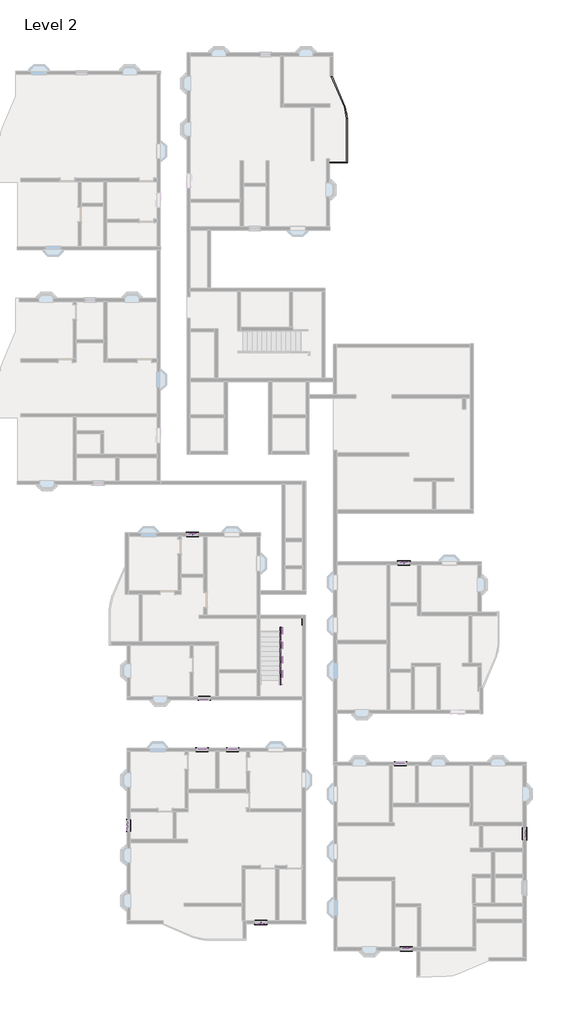
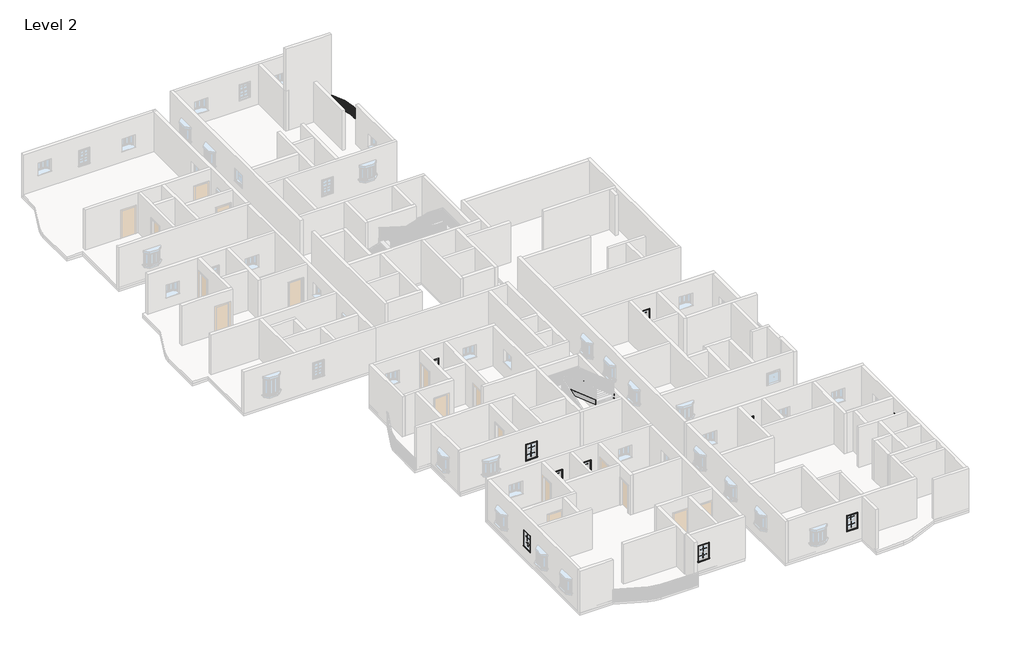
# One storey, part 13 of 14: 40 proxies, 6 members, 1 railing.
"""IFC4 building model written with IfcOpenShell, lengths in millimetres."""

from ifc_helpers import new_model, si_unit, frame, origin, place, context, project, spatial, polyline, circle_curve, outline, extrude, transform, mapped, element, save
from ifc_brep_helpers import plane_surface, cylinder_surface, revolved_surface, advanced_brep
from components import muntin_pattern_2x2_muntin_pattern_2x2_c35c595f, trim_window_exterior_flat_with_sill_e38017c9, trim_window_interior_flat_picture_frame_d728ed12

model = new_model("IFC4")

# Units and contexts
model_context = context("Model", 3, world=origin())
ifc_project = project(units=[si_unit("LENGTHUNIT", "METRE", prefix="MILLI")], contexts=[model_context])

# Site, building, storey
site = spatial("IfcSite", under=ifc_project)
building = spatial("IfcBuilding", under=site)
storey = spatial("IfcBuildingStorey", under=building, Name="Level 2", Elevation=3048.0)

# Proxies
placement = place(None, origin())
muntin_pattern_2x2_muntin_pattern_2x2_shape = muntin_pattern_2x2_muntin_pattern_2x2_c35c595f(model_context)
element("IfcBuildingElementProxy", 1, Name="Muntin Pattern_2x2 : Muntin Pattern_2x2", ObjectType="Muntin Pattern_2x2 : Muntin Pattern_2x2", at=placement, inside=storey, context=model_context, shape_type="MappedRepresentation", body=[
    mapped(muntin_pattern_2x2_muntin_pattern_2x2_shape, transform((-8150.287215, -357.5666506, 4518.025), x_axis=(1.0, 0.0, 0.0), y_axis=(0.0, 1.0, 0.0), z_axis=(0.0, 0.0, 1.0))),
])
element("IfcBuildingElementProxy", 2, Name="Muntin Pattern_2x2 : Muntin Pattern_2x2", ObjectType="Muntin Pattern_2x2 : Muntin Pattern_2x2", at=placement, inside=storey, context=model_context, shape_type="MappedRepresentation", body=[
    mapped(muntin_pattern_2x2_muntin_pattern_2x2_shape, transform((-8150.287215, -402.0166506, 4038.6), x_axis=(1.0, 0.0, 0.0), y_axis=(0.0, 1.0, 0.0), z_axis=(0.0, 0.0, 1.0))),
])
element("IfcBuildingElementProxy", 3, Name="Muntin Pattern_2x2 : Muntin Pattern_2x2", ObjectType="Muntin Pattern_2x2 : Muntin Pattern_2x2", at=placement, inside=storey, context=model_context, shape_type="MappedRepresentation", body=[
    mapped(muntin_pattern_2x2_muntin_pattern_2x2_shape, transform((-7397.812215, -10854.1166506, 4518.025), x_axis=(-1.0, 0.0, 0.0), y_axis=(0.0, -1.0, 0.0), z_axis=(0.0, 0.0, 1.0))),
])
element("IfcBuildingElementProxy", 4, Name="Muntin Pattern_2x2 : Muntin Pattern_2x2", ObjectType="Muntin Pattern_2x2 : Muntin Pattern_2x2", at=placement, inside=storey, context=model_context, shape_type="MappedRepresentation", body=[
    mapped(muntin_pattern_2x2_muntin_pattern_2x2_shape, transform((-7397.812215, -10809.6666506, 4038.6), x_axis=(-1.0, 0.0, 0.0), y_axis=(0.0, -1.0, 0.0), z_axis=(0.0, 0.0, 1.0))),
])
element("IfcBuildingElementProxy", 5, Name="Muntin Pattern_2x2 : Muntin Pattern_2x2", ObjectType="Muntin Pattern_2x2 : Muntin Pattern_2x2", at=placement, inside=storey, context=model_context, shape_type="MappedRepresentation", body=[
    mapped(muntin_pattern_2x2_muntin_pattern_2x2_shape, transform((-7540.687215, -13997.3666506, 4518.025), x_axis=(1.0, 0.0, 0.0), y_axis=(0.0, 1.0, 0.0), z_axis=(0.0, 0.0, 1.0))),
])
element("IfcBuildingElementProxy", 6, Name="Muntin Pattern_2x2 : Muntin Pattern_2x2", ObjectType="Muntin Pattern_2x2 : Muntin Pattern_2x2", at=placement, inside=storey, context=model_context, shape_type="MappedRepresentation", body=[
    mapped(muntin_pattern_2x2_muntin_pattern_2x2_shape, transform((-7540.687215, -14041.8166506, 4038.6), x_axis=(1.0, 0.0, 0.0), y_axis=(0.0, 1.0, 0.0), z_axis=(0.0, 0.0, 1.0))),
])
element("IfcBuildingElementProxy", 7, Name="Muntin Pattern_2x2 : Muntin Pattern_2x2", ObjectType="Muntin Pattern_2x2 : Muntin Pattern_2x2", at=placement, inside=storey, context=model_context, shape_type="MappedRepresentation", body=[
    mapped(muntin_pattern_2x2_muntin_pattern_2x2_shape, transform((-5597.587215, -13997.3666506, 4518.025), x_axis=(1.0, 0.0, 0.0), y_axis=(0.0, 1.0, 0.0), z_axis=(0.0, 0.0, 1.0))),
])
element("IfcBuildingElementProxy", 8, Name="Muntin Pattern_2x2 : Muntin Pattern_2x2", ObjectType="Muntin Pattern_2x2 : Muntin Pattern_2x2", at=placement, inside=storey, context=model_context, shape_type="MappedRepresentation", body=[
    mapped(muntin_pattern_2x2_muntin_pattern_2x2_shape, transform((-5597.587215, -14041.8166506, 4038.6), x_axis=(1.0, 0.0, 0.0), y_axis=(0.0, 1.0, 0.0), z_axis=(0.0, 0.0, 1.0))),
])
element("IfcBuildingElementProxy", 9, Name="Muntin Pattern_2x2 : Muntin Pattern_2x2", ObjectType="Muntin Pattern_2x2 : Muntin Pattern_2x2", at=placement, inside=storey, context=model_context, shape_type="MappedRepresentation", body=[
    mapped(muntin_pattern_2x2_muntin_pattern_2x2_shape, transform((-12255.562215, -18863.6994419, 4518.025), x_axis=(0.0, 1.0, 0.0), y_axis=(-1.0, 0.0, 0.0), z_axis=(0.0, 0.0, 1.0))),
])
element("IfcBuildingElementProxy", 10, Name="Muntin Pattern_2x2 : Muntin Pattern_2x2", ObjectType="Muntin Pattern_2x2 : Muntin Pattern_2x2", at=placement, inside=storey, context=model_context, shape_type="MappedRepresentation", body=[
    mapped(muntin_pattern_2x2_muntin_pattern_2x2_shape, transform((-12211.112215, -18863.6994419, 4038.6), x_axis=(0.0, 1.0, 0.0), y_axis=(-1.0, 0.0, 0.0), z_axis=(0.0, 0.0, 1.0))),
])
element("IfcBuildingElementProxy", 11, Name="Muntin Pattern_2x2 : Muntin Pattern_2x2", ObjectType="Muntin Pattern_2x2 : Muntin Pattern_2x2", at=placement, inside=storey, context=model_context, shape_type="MappedRepresentation", body=[
    mapped(muntin_pattern_2x2_muntin_pattern_2x2_shape, transform((-3806.2891351, -25065.4166506, 4518.025), x_axis=(-1.0, 0.0, 0.0), y_axis=(0.0, -1.0, 0.0), z_axis=(0.0, 0.0, 1.0))),
])
element("IfcBuildingElementProxy", 12, Name="Muntin Pattern_2x2 : Muntin Pattern_2x2", ObjectType="Muntin Pattern_2x2 : Muntin Pattern_2x2", at=placement, inside=storey, context=model_context, shape_type="MappedRepresentation", body=[
    mapped(muntin_pattern_2x2_muntin_pattern_2x2_shape, transform((-3806.2891351, -25020.9666506, 4038.6), x_axis=(-1.0, 0.0, 0.0), y_axis=(0.0, -1.0, 0.0), z_axis=(0.0, 0.0, 1.0))),
])
element("IfcBuildingElementProxy", 13, Name="Muntin Pattern_2x2 : Muntin Pattern_2x2", ObjectType="Muntin Pattern_2x2 : Muntin Pattern_2x2", at=placement, inside=storey, context=model_context, shape_type="MappedRepresentation", body=[
    mapped(muntin_pattern_2x2_muntin_pattern_2x2_shape, transform((5410.0380523, -26615.6292694, 4518.025), x_axis=(1.0, 0.0, 0.0), y_axis=(0.0, 1.0, 0.0), z_axis=(0.0, 0.0, 1.0))),
])
element("IfcBuildingElementProxy", 14, Name="Muntin Pattern_2x2 : Muntin Pattern_2x2", ObjectType="Muntin Pattern_2x2 : Muntin Pattern_2x2", at=placement, inside=storey, context=model_context, shape_type="MappedRepresentation", body=[
    mapped(muntin_pattern_2x2_muntin_pattern_2x2_shape, transform((5410.0380523, -26660.0792694, 4038.6), x_axis=(1.0, 0.0, 0.0), y_axis=(0.0, 1.0, 0.0), z_axis=(0.0, 0.0, 1.0))),
])
element("IfcBuildingElementProxy", 15, Name="Muntin Pattern_2x2 : Muntin Pattern_2x2", ObjectType="Muntin Pattern_2x2 : Muntin Pattern_2x2", at=placement, inside=storey, context=model_context, shape_type="MappedRepresentation", body=[
    mapped(muntin_pattern_2x2_muntin_pattern_2x2_shape, transform((12982.4130523, -19379.8042694, 4518.025), x_axis=(0.0, -1.0, 0.0), y_axis=(1.0, 0.0, 0.0), z_axis=(0.0, 0.0, 1.0))),
])
element("IfcBuildingElementProxy", 16, Name="Muntin Pattern_2x2 : Muntin Pattern_2x2", ObjectType="Muntin Pattern_2x2 : Muntin Pattern_2x2", at=placement, inside=storey, context=model_context, shape_type="MappedRepresentation", body=[
    mapped(muntin_pattern_2x2_muntin_pattern_2x2_shape, transform((12937.9630523, -19379.8042694, 4038.6), x_axis=(0.0, -1.0, 0.0), y_axis=(1.0, 0.0, 0.0), z_axis=(0.0, 0.0, 1.0))),
])
element("IfcBuildingElementProxy", 17, Name="Muntin Pattern_2x2 : Muntin Pattern_2x2", ObjectType="Muntin Pattern_2x2 : Muntin Pattern_2x2", at=placement, inside=storey, context=model_context, shape_type="MappedRepresentation", body=[
    mapped(muntin_pattern_2x2_muntin_pattern_2x2_shape, transform((5048.0880523, -14880.8292694, 4518.025), x_axis=(1.0, 0.0, 0.0), y_axis=(0.0, 1.0, 0.0), z_axis=(0.0, 0.0, 1.0))),
])
element("IfcBuildingElementProxy", 18, Name="Muntin Pattern_2x2 : Muntin Pattern_2x2", ObjectType="Muntin Pattern_2x2 : Muntin Pattern_2x2", at=placement, inside=storey, context=model_context, shape_type="MappedRepresentation", body=[
    mapped(muntin_pattern_2x2_muntin_pattern_2x2_shape, transform((5048.0880523, -14925.2792694, 4038.6), x_axis=(1.0, 0.0, 0.0), y_axis=(0.0, 1.0, 0.0), z_axis=(0.0, 0.0, 1.0))),
])
element("IfcBuildingElementProxy", 19, Name="Muntin Pattern_2x2 : Muntin Pattern_2x2", ObjectType="Muntin Pattern_2x2 : Muntin Pattern_2x2", at=placement, inside=storey, context=model_context, shape_type="MappedRepresentation", body=[
    mapped(muntin_pattern_2x2_muntin_pattern_2x2_shape, transform((5257.6380523, -2168.1292694, 4518.025), x_axis=(1.0, 0.0, 0.0), y_axis=(0.0, 1.0, 0.0), z_axis=(0.0, 0.0, 1.0))),
])
element("IfcBuildingElementProxy", 20, Name="Muntin Pattern_2x2 : Muntin Pattern_2x2", ObjectType="Muntin Pattern_2x2 : Muntin Pattern_2x2", at=placement, inside=storey, context=model_context, shape_type="MappedRepresentation", body=[
    mapped(muntin_pattern_2x2_muntin_pattern_2x2_shape, transform((5257.6380523, -2212.5792694, 4038.6), x_axis=(1.0, 0.0, 0.0), y_axis=(0.0, 1.0, 0.0), z_axis=(0.0, 0.0, 1.0))),
])
trim_window_exterior_flat_with_sill_shape = trim_window_exterior_flat_with_sill_e38017c9(model_context)
element("IfcBuildingElementProxy", 21, Name="Trim-Window-Exterior-Flat : with Sill", ObjectType="Trim-Window-Exterior-Flat : with Sill", at=placement, inside=storey, context=model_context, shape_type="MappedRepresentation", body=[
    mapped(trim_window_exterior_flat_with_sill_shape, transform((-8150.287215, -322.6416506, 5029.2), x_axis=(-1.0, 0.0, 0.0), y_axis=(0.0, 0.0, 1.0), z_axis=(0.0, 1.0, 0.0))),
])
element("IfcBuildingElementProxy", 22, Name="Trim-Window-Exterior-Flat : with Sill", ObjectType="Trim-Window-Exterior-Flat : with Sill", at=placement, inside=storey, context=model_context, shape_type="MappedRepresentation", body=[
    mapped(trim_window_exterior_flat_with_sill_shape, transform((-7397.812215, -10889.0416506, 5029.2), x_axis=(1.0, 0.0, 0.0), y_axis=(0.0, 0.0, 1.0), z_axis=(0.0, -1.0, 0.0))),
])
element("IfcBuildingElementProxy", 23, Name="Trim-Window-Exterior-Flat : with Sill", ObjectType="Trim-Window-Exterior-Flat : with Sill", at=placement, inside=storey, context=model_context, shape_type="MappedRepresentation", body=[
    mapped(trim_window_exterior_flat_with_sill_shape, transform((-7540.687215, -13962.4416506, 5029.2), x_axis=(-1.0, 0.0, 0.0), y_axis=(0.0, 0.0, 1.0), z_axis=(0.0, 1.0, 0.0))),
])
element("IfcBuildingElementProxy", 24, Name="Trim-Window-Exterior-Flat : with Sill", ObjectType="Trim-Window-Exterior-Flat : with Sill", at=placement, inside=storey, context=model_context, shape_type="MappedRepresentation", body=[
    mapped(trim_window_exterior_flat_with_sill_shape, transform((-5597.587215, -13962.4416506, 5029.2), x_axis=(-1.0, 0.0, 0.0), y_axis=(0.0, 0.0, 1.0), z_axis=(0.0, 1.0, 0.0))),
])
element("IfcBuildingElementProxy", 25, Name="Trim-Window-Exterior-Flat : with Sill", ObjectType="Trim-Window-Exterior-Flat : with Sill", at=placement, inside=storey, context=model_context, shape_type="MappedRepresentation", body=[
    mapped(trim_window_exterior_flat_with_sill_shape, transform((-12290.487215, -18863.6994419, 5029.2), x_axis=(0.0, -1.0, 0.0), y_axis=(0.0, 0.0, 1.0), z_axis=(-1.0, 0.0, 0.0))),
])
element("IfcBuildingElementProxy", 26, Name="Trim-Window-Exterior-Flat : with Sill", ObjectType="Trim-Window-Exterior-Flat : with Sill", at=placement, inside=storey, context=model_context, shape_type="MappedRepresentation", body=[
    mapped(trim_window_exterior_flat_with_sill_shape, transform((-3806.2891351, -25100.3416506, 5029.2), x_axis=(1.0, 0.0, 0.0), y_axis=(0.0, 0.0, 1.0), z_axis=(0.0, -1.0, 0.0))),
])
element("IfcBuildingElementProxy", 27, Name="Trim-Window-Exterior-Flat : with Sill", ObjectType="Trim-Window-Exterior-Flat : with Sill", at=placement, inside=storey, context=model_context, shape_type="MappedRepresentation", body=[
    mapped(trim_window_exterior_flat_with_sill_shape, transform((5410.0380523, -26580.7042694, 5029.2), x_axis=(-1.0, 0.0, 0.0), y_axis=(0.0, 0.0, 1.0), z_axis=(0.0, 1.0, 0.0))),
])
element("IfcBuildingElementProxy", 28, Name="Trim-Window-Exterior-Flat : with Sill", ObjectType="Trim-Window-Exterior-Flat : with Sill", at=placement, inside=storey, context=model_context, shape_type="MappedRepresentation", body=[
    mapped(trim_window_exterior_flat_with_sill_shape, transform((13017.3380523, -19379.8042694, 5029.2), x_axis=(0.0, 1.0, 0.0), y_axis=(0.0, 0.0, 1.0), z_axis=(1.0, 0.0, 0.0))),
])
element("IfcBuildingElementProxy", 29, Name="Trim-Window-Exterior-Flat : with Sill", ObjectType="Trim-Window-Exterior-Flat : with Sill", at=placement, inside=storey, context=model_context, shape_type="MappedRepresentation", body=[
    mapped(trim_window_exterior_flat_with_sill_shape, transform((5048.0880523, -14845.9042694, 5029.2), x_axis=(-1.0, 0.0, 0.0), y_axis=(0.0, 0.0, 1.0), z_axis=(0.0, 1.0, 0.0))),
])
element("IfcBuildingElementProxy", 30, Name="Trim-Window-Exterior-Flat : with Sill", ObjectType="Trim-Window-Exterior-Flat : with Sill", at=placement, inside=storey, context=model_context, shape_type="MappedRepresentation", body=[
    mapped(trim_window_exterior_flat_with_sill_shape, transform((5257.6380523, -2133.2042694, 5029.2), x_axis=(-1.0, 0.0, 0.0), y_axis=(0.0, 0.0, 1.0), z_axis=(0.0, 1.0, 0.0))),
])
trim_window_interior_flat_picture_frame_shape = trim_window_interior_flat_picture_frame_d728ed12(model_context)
element("IfcBuildingElementProxy", 31, Name="Trim-Window-Interior-Flat : Picture Frame", ObjectType="Trim-Window-Interior-Flat : Picture Frame", at=placement, inside=storey, context=model_context, shape_type="MappedRepresentation", body=[
    mapped(trim_window_interior_flat_picture_frame_shape, transform((-8150.287215, -525.8416506, 5029.2), x_axis=(1.0, 0.0, 0.0), y_axis=(0.0, 0.0, 1.0), z_axis=(0.0, -1.0, 0.0))),
])
element("IfcBuildingElementProxy", 32, Name="Trim-Window-Interior-Flat : Picture Frame", ObjectType="Trim-Window-Interior-Flat : Picture Frame", at=placement, inside=storey, context=model_context, shape_type="MappedRepresentation", body=[
    mapped(trim_window_interior_flat_picture_frame_shape, transform((-7397.812215, -10685.8416506, 5029.2), x_axis=(-1.0, 0.0, 0.0), y_axis=(0.0, 0.0, 1.0), z_axis=(0.0, 1.0, 0.0))),
])
element("IfcBuildingElementProxy", 33, Name="Trim-Window-Interior-Flat : Picture Frame", ObjectType="Trim-Window-Interior-Flat : Picture Frame", at=placement, inside=storey, context=model_context, shape_type="MappedRepresentation", body=[
    mapped(trim_window_interior_flat_picture_frame_shape, transform((-7540.687215, -14165.6416506, 5029.2), x_axis=(1.0, 0.0, 0.0), y_axis=(0.0, 0.0, 1.0), z_axis=(0.0, -1.0, 0.0))),
])
element("IfcBuildingElementProxy", 34, Name="Trim-Window-Interior-Flat : Picture Frame", ObjectType="Trim-Window-Interior-Flat : Picture Frame", at=placement, inside=storey, context=model_context, shape_type="MappedRepresentation", body=[
    mapped(trim_window_interior_flat_picture_frame_shape, transform((-5597.587215, -14165.6416506, 5029.2), x_axis=(1.0, 0.0, 0.0), y_axis=(0.0, 0.0, 1.0), z_axis=(0.0, -1.0, 0.0))),
])
element("IfcBuildingElementProxy", 35, Name="Trim-Window-Interior-Flat : Picture Frame", ObjectType="Trim-Window-Interior-Flat : Picture Frame", at=placement, inside=storey, context=model_context, shape_type="MappedRepresentation", body=[
    mapped(trim_window_interior_flat_picture_frame_shape, transform((-12087.287215, -18863.6994419, 5029.2), x_axis=(0.0, 1.0, 0.0), y_axis=(0.0, 0.0, 1.0), z_axis=(1.0, 0.0, 0.0))),
])
element("IfcBuildingElementProxy", 36, Name="Trim-Window-Interior-Flat : Picture Frame", ObjectType="Trim-Window-Interior-Flat : Picture Frame", at=placement, inside=storey, context=model_context, shape_type="MappedRepresentation", body=[
    mapped(trim_window_interior_flat_picture_frame_shape, transform((-3806.2891351, -24897.1416506, 5029.2), x_axis=(-1.0, 0.0, 0.0), y_axis=(0.0, 0.0, 1.0), z_axis=(0.0, 1.0, 0.0))),
])
element("IfcBuildingElementProxy", 37, Name="Trim-Window-Interior-Flat : Picture Frame", ObjectType="Trim-Window-Interior-Flat : Picture Frame", at=placement, inside=storey, context=model_context, shape_type="MappedRepresentation", body=[
    mapped(trim_window_interior_flat_picture_frame_shape, transform((5410.0380523, -26783.9042694, 5029.2), x_axis=(1.0, 0.0, 0.0), y_axis=(0.0, 0.0, 1.0), z_axis=(0.0, -1.0, 0.0))),
])
element("IfcBuildingElementProxy", 38, Name="Trim-Window-Interior-Flat : Picture Frame", ObjectType="Trim-Window-Interior-Flat : Picture Frame", at=placement, inside=storey, context=model_context, shape_type="MappedRepresentation", body=[
    mapped(trim_window_interior_flat_picture_frame_shape, transform((12814.1380523, -19379.8042694, 5029.2), x_axis=(0.0, -1.0, 0.0), y_axis=(0.0, 0.0, 1.0), z_axis=(-1.0, 0.0, 0.0))),
])
element("IfcBuildingElementProxy", 39, Name="Trim-Window-Interior-Flat : Picture Frame", ObjectType="Trim-Window-Interior-Flat : Picture Frame", at=placement, inside=storey, context=model_context, shape_type="MappedRepresentation", body=[
    mapped(trim_window_interior_flat_picture_frame_shape, transform((5048.0880523, -15049.1042694, 5029.2), x_axis=(1.0, 0.0, 0.0), y_axis=(0.0, 0.0, 1.0), z_axis=(0.0, -1.0, 0.0))),
])
element("IfcBuildingElementProxy", 40, Name="Trim-Window-Interior-Flat : Picture Frame", ObjectType="Trim-Window-Interior-Flat : Picture Frame", at=placement, inside=storey, context=model_context, shape_type="MappedRepresentation", body=[
    mapped(trim_window_interior_flat_picture_frame_shape, transform((5257.6380523, -2336.4042694, 5029.2), x_axis=(1.0, 0.0, 0.0), y_axis=(0.0, 0.0, 1.0), z_axis=(0.0, -1.0, 0.0))),
])

# Members
element("IfcMember", 41, ObjectType="Stringer - 2\" Width", at=placement, inside=storey, context=model_context, shape_type="SweptSolid", body=[
    extrude(outline(polyline([(-9955.5916506, 3048.0), (-9955.5916506, 3239.3592169), (-6325.8738327, 4495.8), (-5713.7916506, 4495.8), (-5713.7916506, 4385.1301656), (-9576.612129, 3048.0), (-9955.5916506, 3048.0)])), frame((-3908.487215, 0.0, 0.0), z_axis=(1.0, 0.0, 0.0), x_axis=(0.0, 1.0, 0.0)), (0.0, 0.0, 1.0), 50.8),
])
element("IfcMember", 42, ObjectType="Stringer - 2\" Width", at=placement, inside=storey, context=model_context, shape_type="SweptSolid", body=[
    extrude(outline(polyline([(-3908.487215, -5713.7916506), (-3908.487215, -5662.9916506), (-1190.687215, -5662.9916506), (-1190.687215, -5713.7916506), (-3908.487215, -5713.7916506)])), frame((0.0, 0.0, 4191.0), z_axis=(0.0, 0.0, 1.0), x_axis=(1.0, 0.0, 0.0)), (0.0, 0.0, 1.0), 304.8),
])
element("IfcMember", 43, ObjectType="Stringer - 2\" Width", at=placement, inside=storey, context=model_context, shape_type="SweptSolid", body=[
    extrude(outline(polyline([(-5662.9916506, 4395.5476784), (-5662.9916506, 4191.0), (-6003.8711722, 4191.0), (-9949.2416506, 5556.7051656), (-9949.2416506, 5879.2496015), (-5662.9916506, 4395.5476784)])), frame((-1190.687215, 0.0, 0.0), z_axis=(1.0, 0.0, 0.0), x_axis=(0.0, 1.0, 0.0)), (0.0, 0.0, 1.0), 50.8),
])
element("IfcMember", 44, ObjectType="Stringer - 2\" Width", at=placement, inside=storey, context=model_context, shape_type="SweptSolid", body=[
    extrude(outline(polyline([(-9955.5916506, 3048.0), (-9955.5916506, 3239.3592169), (-6342.4416506, 4490.0649861), (-6342.4416506, 4167.5205502), (-9576.612129, 3048.0), (-9955.5916506, 3048.0)])), frame((-2593.7381751, 0.0, 0.0), z_axis=(1.0, 0.0, 0.0), x_axis=(0.0, 1.0, 0.0)), (0.0, 0.0, 1.0), 50.8),
])
element("IfcMember", 45, ObjectType="Stringer - 2\" Width", at=placement, inside=storey, context=model_context, shape_type="SweptSolid", body=[
    extrude(outline(polyline([(-2593.7381751, -6342.4416506), (-2593.7381751, -6291.6416506), (-2492.1381751, -6291.6416506), (-2492.1381751, -6342.4416506), (-2593.7381751, -6342.4416506)])), frame((0.0, 0.0, 4191.0), z_axis=(0.0, 0.0, 1.0), x_axis=(1.0, 0.0, 0.0)), (0.0, 0.0, 1.0), 304.8),
])
element("IfcMember", 46, ObjectType="Stringer - 2\" Width", at=placement, inside=storey, context=model_context, shape_type="SweptSolid", body=[
    extrude(outline(polyline([(-6291.6416506, 4613.1572938), (-6291.6416506, 4290.6128579), (-9949.2416506, 5556.7051656), (-9949.2416506, 5879.2496015), (-6291.6416506, 4613.1572938)])), frame((-2492.1381751, 0.0, 0.0), z_axis=(1.0, 0.0, 0.0), x_axis=(0.0, 1.0, 0.0)), (0.0, 0.0, 1.0), 50.8),
])

# Railing
element("IfcRailing", 47, ObjectType="Handrail - Rectangular", at=placement, inside=storey, context=model_context, shape_type="SolidModel", body=[
    advanced_brep(
    [(549.8108649, 23180.4215905, 3962.4), (549.8108649, 23180.4215905, 3911.6), (549.8108649, 23129.6215905, 3911.6), (549.8108649, 23129.6215905, 3962.4), (1629.3108649, 23180.4215905, 3962.4), (1629.3108649, 23180.4215905, 3911.6), (1680.1108649, 23129.6215905, 3911.6), (1680.1108649, 23129.6215905, 3962.4), (1629.3108649, 25921.9580583, 3962.4), (1629.3108649, 25921.9580583, 3911.6), (1680.1108649, 25921.9580583, 3911.6), (1680.1108649, 25921.9580583, 3962.4), (1475.5051478, 26671.8537734, 3911.6), (1475.5051478, 26671.8537734, 3962.4), (1522.203662, 26691.8509925, 3911.6), (1522.203662, 26691.8509925, 3962.4), (640.7616078, 28621.188975, 3962.4), (687.460122, 28641.186194, 3962.4), (687.460122, 28641.186194, 3911.6), (640.7616078, 28621.188975, 3911.6)],
    [
        (0, 1),
        (1, 2),
        (2, 3),
        (3, 0),
        (0, 4),
        (4, 5),
        (5, 1),
        (5, 6),
        (6, 2),
        (6, 7),
        (7, 3),
        (7, 4),
        (4, 8),
        (8, 9),
        (9, 5),
        (9, 10),
        (10, 6),
        (10, 11),
        (11, 7),
        (11, 8),
        (12, 9, circle_curve(frame((-275.6891351, 25921.9580583, 3911.6), z_axis=(0.0, 0.0, -1.0), x_axis=(1.0, 0.0, 0.0)), 1905.0)),
        (8, 13, circle_curve(frame((-275.6891351, 25921.9580583, 3962.4), z_axis=(0.0, 0.0, 1.0), x_axis=(1.0, 0.0, 0.0)), 1905.0)),
        (13, 12),
        (14, 10, circle_curve(frame((-275.6891351, 25921.9580583, 3911.6), z_axis=(0.0, 0.0, -1.0), x_axis=(1.0, 0.0, 0.0)), 1955.8)),
        (12, 14),
        (15, 11, circle_curve(frame((-275.6891351, 25921.9580583, 3962.4), z_axis=(0.0, 0.0, -1.0), x_axis=(1.0, 0.0, 0.0)), 1955.8)),
        (14, 15),
        (15, 13),
        (16, 17),
        (17, 18),
        (18, 19),
        (19, 16),
        (13, 16),
        (19, 12),
        (18, 14),
        (17, 15),
    ],
    [
        plane_surface(frame((549.8108649, 23155.0215905, 3962.4), z_axis=(-1.0, 0.0, 0.0), x_axis=(0.0, 1.0, 0.0))),
        plane_surface(frame((549.8108649, 23180.4215905, 3962.4), z_axis=(0.0, 1.0, 0.0), x_axis=(1.0, 0.0, 0.0))),
        plane_surface(frame((549.8108649, 23180.4215905, 3911.6), z_axis=(0.0, 0.0, -1.0), x_axis=(1.0, 0.0, 0.0))),
        plane_surface(frame((549.8108649, 23129.6215905, 3911.6), z_axis=(0.0, -1.0, 0.0), x_axis=(1.0, 0.0, 0.0))),
        plane_surface(frame((549.8108649, 23129.6215905, 3962.4), z_axis=(0.0, 0.0, 1.0), x_axis=(1.0, 0.0, 0.0))),
        plane_surface(frame((1629.3108649, 23180.4215905, 3962.4), z_axis=(-1.0, 0.0, 0.0), x_axis=(0.0, 1.0, 0.0))),
        plane_surface(frame((1629.3108649, 23180.4215905, 3911.6), z_axis=(0.0, 0.0, -1.0), x_axis=(0.0, 1.0, 0.0))),
        plane_surface(frame((1680.1108649, 23129.6215905, 3911.6), z_axis=(1.0, 0.0, 0.0), x_axis=(0.0, 1.0, 0.0))),
        plane_surface(frame((1680.1108649, 23129.6215905, 3962.4), z_axis=(0.0, 0.0, 1.0), x_axis=(0.0, 1.0, 0.0))),
        revolved_surface(polyline([(1629.3108649, 25921.9580583, 3962.4), (1629.3108649, 25921.9580583, 3911.6)]), (-275.6891351, 25921.9580583, 3962.4), (0.0, 0.0, 1.0)),
        plane_surface(frame((-275.6891351, 25921.9580583, 3911.6), z_axis=(0.0, 0.0, -1.0), x_axis=(1.0, 0.0, 0.0))),
        cylinder_surface(frame((-275.6891351, 25921.9580583, 3962.4), z_axis=(0.0, 0.0, 1.0), x_axis=(1.0, 0.0, 0.0)), 1955.8),
        plane_surface(frame((-275.6891351, 25921.9580583, 3962.4), z_axis=(0.0, 0.0, 1.0), x_axis=(1.0, 0.0, 0.0))),
        plane_surface(frame((664.1108649, 28631.1875845, 3962.4), z_axis=(-0.39364604467361036, 0.91926209076238, 0.0), x_axis=(0.91926209076238, 0.39364604467361036, 0.0))),
        plane_surface(frame((1475.5051478, 26671.8537734, 3962.4), z_axis=(-0.9192620907623801, -0.39364604467361014, 0.0), x_axis=(-0.39364604467361014, 0.9192620907623801, 0.0))),
        plane_surface(frame((1475.5051478, 26671.8537734, 3911.6), z_axis=(0.0, 0.0, -1.0000000000000002), x_axis=(-0.39364604467361014, 0.9192620907623801, 0.0))),
        plane_surface(frame((1522.203662, 26691.8509925, 3911.6), z_axis=(0.91926209076238, 0.39364604467361014, 0.0), x_axis=(-0.39364604467361014, 0.91926209076238, 0.0))),
        plane_surface(frame((1522.203662, 26691.8509925, 3962.4), z_axis=(0.0, 0.0, 1.0), x_axis=(-0.39364604467361014, 0.91926209076238, 0.0))),
    ],
    [
        (0, [[1, 2, 3, 4]]),
        (1, [[-1, 5, 6, 7]]),
        (2, [[-2, -7, 8, 9]]),
        (3, [[-3, -9, 10, 11]]),
        (4, [[-4, -11, 12, -5]]),
        (5, [[-6, 13, 14, 15]]),
        (6, [[-8, -15, 16, 17]]),
        (7, [[-10, -17, 18, 19]]),
        (8, [[-12, -19, 20, -13]]),
        (9, [[21, -14, 22, 23]]),
        (10, [[24, -16, -21, 25]]),
        (11, [[26, -18, -24, 27]]),
        (12, [[-22, -20, -26, 28]]),
        (13, [[29, 30, 31, 32]]),
        (14, [[-23, 33, -32, 34]]),
        (15, [[-25, -34, -31, 35]]),
        (16, [[-27, -35, -30, 36]]),
        (17, [[-28, -36, -29, -33]]),
    ],
),
    extrude(outline(polyline([(711.4710921, 28544.7864585), (693.9591493, 28537.2875014), (686.4601921, 28554.7994442), (703.9721349, 28562.2984014), (711.4710921, 28544.7864585)])), frame((0.0, 0.0, 3048.0), z_axis=(0.0, 0.0, 1.0), x_axis=(1.0, 0.0, 0.0)), (0.0, 0.0, 1.0), 863.6),
    extrude(outline(polyline([(751.4655302, 28451.3894301), (733.9535874, 28443.890473), (726.4546303, 28461.4024158), (743.9665731, 28468.9013729), (751.4655302, 28451.3894301)])), frame((0.0, 0.0, 3048.0), z_axis=(0.0, 0.0, 1.0), x_axis=(1.0, 0.0, 0.0)), (0.0, 0.0, 1.0), 863.6),
    extrude(outline(polyline([(791.4599684, 28357.9924017), (773.9480255, 28350.4934445), (766.4490684, 28368.0053874), (783.9610112, 28375.5043445), (791.4599684, 28357.9924017)])), frame((0.0, 0.0, 3048.0), z_axis=(0.0, 0.0, 1.0), x_axis=(1.0, 0.0, 0.0)), (0.0, 0.0, 1.0), 863.6),
    extrude(outline(polyline([(831.4544065, 28264.5953733), (813.9424637, 28257.0964161), (806.4435065, 28274.608359), (823.9554494, 28282.1073161), (831.4544065, 28264.5953733)])), frame((0.0, 0.0, 3048.0), z_axis=(0.0, 0.0, 1.0), x_axis=(1.0, 0.0, 0.0)), (0.0, 0.0, 1.0), 863.6),
    extrude(outline(polyline([(871.4488446, 28171.1983449), (853.9369018, 28163.6993877), (846.4379447, 28181.2113305), (863.9498875, 28188.7102877), (871.4488446, 28171.1983449)])), frame((0.0, 0.0, 3048.0), z_axis=(0.0, 0.0, 1.0), x_axis=(1.0, 0.0, 0.0)), (0.0, 0.0, 1.0), 863.6),
    extrude(outline(polyline([(911.4432828, 28077.8013164), (893.93134, 28070.3023593), (886.4323828, 28087.8143021), (903.9443256, 28095.3132593), (911.4432828, 28077.8013164)])), frame((0.0, 0.0, 3048.0), z_axis=(0.0, 0.0, 1.0), x_axis=(1.0, 0.0, 0.0)), (0.0, 0.0, 1.0), 863.6),
    extrude(outline(polyline([(951.4377209, 27984.404288), (933.9257781, 27976.9053309), (926.4268209, 27994.4172737), (943.9387638, 28001.9162308), (951.4377209, 27984.404288)])), frame((0.0, 0.0, 3048.0), z_axis=(0.0, 0.0, 1.0), x_axis=(1.0, 0.0, 0.0)), (0.0, 0.0, 1.0), 863.6),
    extrude(outline(polyline([(991.4321591, 27891.0072596), (973.9202162, 27883.5083024), (966.4212591, 27901.0202453), (983.9332019, 27908.5192024), (991.4321591, 27891.0072596)])), frame((0.0, 0.0, 3048.0), z_axis=(0.0, 0.0, 1.0), x_axis=(1.0, 0.0, 0.0)), (0.0, 0.0, 1.0), 863.6),
    extrude(outline(polyline([(1031.4265972, 27797.6102312), (1013.9146544, 27790.111274), (1006.4156972, 27807.6232168), (1023.9276401, 27815.122174), (1031.4265972, 27797.6102312)])), frame((0.0, 0.0, 3048.0), z_axis=(0.0, 0.0, 1.0), x_axis=(1.0, 0.0, 0.0)), (0.0, 0.0, 1.0), 863.6),
    extrude(outline(polyline([(1071.4210353, 27704.2132027), (1053.9090925, 27696.7142456), (1046.4101354, 27714.2261884), (1063.9220782, 27721.7251456), (1071.4210353, 27704.2132027)])), frame((0.0, 0.0, 3048.0), z_axis=(0.0, 0.0, 1.0), x_axis=(1.0, 0.0, 0.0)), (0.0, 0.0, 1.0), 863.6),
    extrude(outline(polyline([(1111.4154735, 27610.8161743), (1093.9035307, 27603.3172172), (1086.4045735, 27620.82916), (1103.9165163, 27628.3281172), (1111.4154735, 27610.8161743)])), frame((0.0, 0.0, 3048.0), z_axis=(0.0, 0.0, 1.0), x_axis=(1.0, 0.0, 0.0)), (0.0, 0.0, 1.0), 863.6),
    extrude(outline(polyline([(1151.4099116, 27517.4191459), (1133.8979688, 27509.9201888), (1126.3990116, 27527.4321316), (1143.9109545, 27534.9310887), (1151.4099116, 27517.4191459)])), frame((0.0, 0.0, 3048.0), z_axis=(0.0, 0.0, 1.0), x_axis=(1.0, 0.0, 0.0)), (0.0, 0.0, 1.0), 863.6),
    extrude(outline(polyline([(1191.4043498, 27424.0221175), (1173.8924069, 27416.5231603), (1166.3934498, 27434.0351032), (1183.9053926, 27441.5340603), (1191.4043498, 27424.0221175)])), frame((0.0, 0.0, 3048.0), z_axis=(0.0, 0.0, 1.0), x_axis=(1.0, 0.0, 0.0)), (0.0, 0.0, 1.0), 863.6),
    extrude(outline(polyline([(1231.3987879, 27330.6250891), (1213.8868451, 27323.1261319), (1206.3878879, 27340.6380747), (1223.8998307, 27348.1370319), (1231.3987879, 27330.6250891)])), frame((0.0, 0.0, 3048.0), z_axis=(0.0, 0.0, 1.0), x_axis=(1.0, 0.0, 0.0)), (0.0, 0.0, 1.0), 863.6),
    extrude(outline(polyline([(1271.393226, 27237.2280606), (1253.8812832, 27229.7291035), (1246.3823261, 27247.2410463), (1263.8942689, 27254.7400035), (1271.393226, 27237.2280606)])), frame((0.0, 0.0, 3048.0), z_axis=(0.0, 0.0, 1.0), x_axis=(1.0, 0.0, 0.0)), (0.0, 0.0, 1.0), 863.6),
    extrude(outline(polyline([(1311.3876642, 27143.8310322), (1293.8757213, 27136.3320751), (1286.3767642, 27153.8440179), (1303.888707, 27161.342975), (1311.3876642, 27143.8310322)])), frame((0.0, 0.0, 3048.0), z_axis=(0.0, 0.0, 1.0), x_axis=(1.0, 0.0, 0.0)), (0.0, 0.0, 1.0), 863.6),
    extrude(outline(polyline([(1351.3821023, 27050.4340038), (1333.8701595, 27042.9350466), (1326.3712023, 27060.4469895), (1343.8831452, 27067.9459466), (1351.3821023, 27050.4340038)])), frame((0.0, 0.0, 3048.0), z_axis=(0.0, 0.0, 1.0), x_axis=(1.0, 0.0, 0.0)), (0.0, 0.0, 1.0), 863.6),
    extrude(outline(polyline([(1391.3765405, 26957.0369754), (1373.8645976, 26949.5380182), (1366.3656405, 26967.0499611), (1383.8775833, 26974.5489182), (1391.3765405, 26957.0369754)])), frame((0.0, 0.0, 3048.0), z_axis=(0.0, 0.0, 1.0), x_axis=(1.0, 0.0, 0.0)), (0.0, 0.0, 1.0), 863.6),
    extrude(outline(polyline([(1431.3709786, 26863.639947), (1413.8590358, 26856.1409898), (1406.3600786, 26873.6529326), (1423.8720214, 26881.1518898), (1431.3709786, 26863.639947)])), frame((0.0, 0.0, 3048.0), z_axis=(0.0, 0.0, 1.0), x_axis=(1.0, 0.0, 0.0)), (0.0, 0.0, 1.0), 863.6),
    extrude(outline(polyline([(1471.3654167, 26770.2429185), (1453.8534739, 26762.7439614), (1446.3545168, 26780.2559042), (1463.8664596, 26787.7548614), (1471.3654167, 26770.2429185)])), frame((0.0, 0.0, 3048.0), z_axis=(0.0, 0.0, 1.0), x_axis=(1.0, 0.0, 0.0)), (0.0, 0.0, 1.0), 863.6),
    extrude(outline(polyline([(1537.4917391, 26611.722401), (1519.7200483, 26604.8616791), (1512.8593263, 26622.6333699), (1530.6310171, 26629.4940918), (1537.4917391, 26611.722401)])), frame((0.0, 0.0, 3048.0), z_axis=(0.0, 0.0, 1.0), x_axis=(1.0, 0.0, 0.0)), (0.0, 0.0, 1.0), 863.6),
    extrude(outline(polyline([(1571.2676162, 26515.3807493), (1553.1596103, 26509.4644479), (1547.2433088, 26527.5724538), (1565.3513147, 26533.4887552), (1571.2676162, 26515.3807493)])), frame((0.0, 0.0, 3048.0), z_axis=(0.0, 0.0, 1.0), x_axis=(1.0, 0.0, 0.0)), (0.0, 0.0, 1.0), 863.6),
    extrude(outline(polyline([(1599.9284504, 26417.3956468), (1581.5342785, 26412.4401508), (1576.5787825, 26430.8343227), (1594.9729544, 26435.7898187), (1599.9284504, 26417.3956468)])), frame((0.0, 0.0, 3048.0), z_axis=(0.0, 0.0, 1.0), x_axis=(1.0, 0.0, 0.0)), (0.0, 0.0, 1.0), 863.6),
    extrude(outline(polyline([(1623.3948673, 26318.0384578), (1604.7654711, 26314.0574912), (1600.7845045, 26332.6868874), (1619.4139008, 26336.667854), (1623.3948673, 26318.0384578)])), frame((0.0, 0.0, 3048.0), z_axis=(0.0, 0.0, 1.0), x_axis=(1.0, 0.0, 0.0)), (0.0, 0.0, 1.0), 863.6),
    extrude(outline(polyline([(1641.601878, 26217.5843464), (1622.7888504, 26214.5889343), (1619.7934383, 26233.4019618), (1638.6064659, 26236.3973739), (1641.601878, 26217.5843464)])), frame((0.0, 0.0, 3048.0), z_axis=(0.0, 0.0, 1.0), x_axis=(1.0, 0.0, 0.0)), (0.0, 0.0, 1.0), 863.6),
    extrude(outline(polyline([(1654.4990591, 26116.3115146), (1635.5545019, 26114.3099526), (1633.5529398, 26133.2545098), (1652.4974971, 26135.2560719), (1654.4990591, 26116.3115146)])), frame((0.0, 0.0, 3048.0), z_axis=(0.0, 0.0, 1.0), x_axis=(1.0, 0.0, 0.0)), (0.0, 0.0, 1.0), 863.6),
    extrude(outline(polyline([(1662.0506927, 26014.5004319), (1643.0270716, 26013.4982632), (1642.0249029, 26032.5218842), (1661.048524, 26033.524053), (1662.0506927, 26014.5004319)])), frame((0.0, 0.0, 3048.0), z_axis=(0.0, 0.0, 1.0), x_axis=(1.0, 0.0, 0.0)), (0.0, 0.0, 1.0), 863.6),
    extrude(outline(polyline([(1664.2358649, 25888.6965905), (1645.1858649, 25888.6965905), (1645.1858649, 25907.7465905), (1664.2358649, 25907.7465905), (1664.2358649, 25888.6965905)])), frame((0.0, 0.0, 3048.0), z_axis=(0.0, 0.0, 1.0), x_axis=(1.0, 0.0, 0.0)), (0.0, 0.0, 1.0), 863.6),
    extrude(outline(polyline([(1664.2358649, 25787.0965905), (1645.1858649, 25787.0965905), (1645.1858649, 25806.1465905), (1664.2358649, 25806.1465905), (1664.2358649, 25787.0965905)])), frame((0.0, 0.0, 3048.0), z_axis=(0.0, 0.0, 1.0), x_axis=(1.0, 0.0, 0.0)), (0.0, 0.0, 1.0), 863.6),
    extrude(outline(polyline([(1664.2358649, 25685.4965905), (1645.1858649, 25685.4965905), (1645.1858649, 25704.5465905), (1664.2358649, 25704.5465905), (1664.2358649, 25685.4965905)])), frame((0.0, 0.0, 3048.0), z_axis=(0.0, 0.0, 1.0), x_axis=(1.0, 0.0, 0.0)), (0.0, 0.0, 1.0), 863.6),
    extrude(outline(polyline([(1664.2358649, 25583.8965905), (1645.1858649, 25583.8965905), (1645.1858649, 25602.9465905), (1664.2358649, 25602.9465905), (1664.2358649, 25583.8965905)])), frame((0.0, 0.0, 3048.0), z_axis=(0.0, 0.0, 1.0), x_axis=(1.0, 0.0, 0.0)), (0.0, 0.0, 1.0), 863.6),
    extrude(outline(polyline([(1664.2358649, 25482.2965905), (1645.1858649, 25482.2965905), (1645.1858649, 25501.3465905), (1664.2358649, 25501.3465905), (1664.2358649, 25482.2965905)])), frame((0.0, 0.0, 3048.0), z_axis=(0.0, 0.0, 1.0), x_axis=(1.0, 0.0, 0.0)), (0.0, 0.0, 1.0), 863.6),
    extrude(outline(polyline([(1664.2358649, 25380.6965905), (1645.1858649, 25380.6965905), (1645.1858649, 25399.7465905), (1664.2358649, 25399.7465905), (1664.2358649, 25380.6965905)])), frame((0.0, 0.0, 3048.0), z_axis=(0.0, 0.0, 1.0), x_axis=(1.0, 0.0, 0.0)), (0.0, 0.0, 1.0), 863.6),
    extrude(outline(polyline([(1664.2358649, 25279.0965905), (1645.1858649, 25279.0965905), (1645.1858649, 25298.1465905), (1664.2358649, 25298.1465905), (1664.2358649, 25279.0965905)])), frame((0.0, 0.0, 3048.0), z_axis=(0.0, 0.0, 1.0), x_axis=(1.0, 0.0, 0.0)), (0.0, 0.0, 1.0), 863.6),
    extrude(outline(polyline([(1664.2358649, 25177.4965905), (1645.1858649, 25177.4965905), (1645.1858649, 25196.5465905), (1664.2358649, 25196.5465905), (1664.2358649, 25177.4965905)])), frame((0.0, 0.0, 3048.0), z_axis=(0.0, 0.0, 1.0), x_axis=(1.0, 0.0, 0.0)), (0.0, 0.0, 1.0), 863.6),
    extrude(outline(polyline([(1664.2358649, 25075.8965905), (1645.1858649, 25075.8965905), (1645.1858649, 25094.9465905), (1664.2358649, 25094.9465905), (1664.2358649, 25075.8965905)])), frame((0.0, 0.0, 3048.0), z_axis=(0.0, 0.0, 1.0), x_axis=(1.0, 0.0, 0.0)), (0.0, 0.0, 1.0), 863.6),
    extrude(outline(polyline([(1664.2358649, 24974.2965905), (1645.1858649, 24974.2965905), (1645.1858649, 24993.3465905), (1664.2358649, 24993.3465905), (1664.2358649, 24974.2965905)])), frame((0.0, 0.0, 3048.0), z_axis=(0.0, 0.0, 1.0), x_axis=(1.0, 0.0, 0.0)), (0.0, 0.0, 1.0), 863.6),
    extrude(outline(polyline([(1664.2358649, 24872.6965905), (1645.1858649, 24872.6965905), (1645.1858649, 24891.7465905), (1664.2358649, 24891.7465905), (1664.2358649, 24872.6965905)])), frame((0.0, 0.0, 3048.0), z_axis=(0.0, 0.0, 1.0), x_axis=(1.0, 0.0, 0.0)), (0.0, 0.0, 1.0), 863.6),
    extrude(outline(polyline([(1664.2358649, 24771.0965905), (1645.1858649, 24771.0965905), (1645.1858649, 24790.1465905), (1664.2358649, 24790.1465905), (1664.2358649, 24771.0965905)])), frame((0.0, 0.0, 3048.0), z_axis=(0.0, 0.0, 1.0), x_axis=(1.0, 0.0, 0.0)), (0.0, 0.0, 1.0), 863.6),
    extrude(outline(polyline([(1664.2358649, 24669.4965905), (1645.1858649, 24669.4965905), (1645.1858649, 24688.5465905), (1664.2358649, 24688.5465905), (1664.2358649, 24669.4965905)])), frame((0.0, 0.0, 3048.0), z_axis=(0.0, 0.0, 1.0), x_axis=(1.0, 0.0, 0.0)), (0.0, 0.0, 1.0), 863.6),
    extrude(outline(polyline([(1664.2358649, 24567.8965905), (1645.1858649, 24567.8965905), (1645.1858649, 24586.9465905), (1664.2358649, 24586.9465905), (1664.2358649, 24567.8965905)])), frame((0.0, 0.0, 3048.0), z_axis=(0.0, 0.0, 1.0), x_axis=(1.0, 0.0, 0.0)), (0.0, 0.0, 1.0), 863.6),
    extrude(outline(polyline([(1664.2358649, 24466.2965905), (1645.1858649, 24466.2965905), (1645.1858649, 24485.3465905), (1664.2358649, 24485.3465905), (1664.2358649, 24466.2965905)])), frame((0.0, 0.0, 3048.0), z_axis=(0.0, 0.0, 1.0), x_axis=(1.0, 0.0, 0.0)), (0.0, 0.0, 1.0), 863.6),
    extrude(outline(polyline([(1664.2358649, 24364.6965905), (1645.1858649, 24364.6965905), (1645.1858649, 24383.7465905), (1664.2358649, 24383.7465905), (1664.2358649, 24364.6965905)])), frame((0.0, 0.0, 3048.0), z_axis=(0.0, 0.0, 1.0), x_axis=(1.0, 0.0, 0.0)), (0.0, 0.0, 1.0), 863.6),
    extrude(outline(polyline([(1664.2358649, 24263.0965905), (1645.1858649, 24263.0965905), (1645.1858649, 24282.1465905), (1664.2358649, 24282.1465905), (1664.2358649, 24263.0965905)])), frame((0.0, 0.0, 3048.0), z_axis=(0.0, 0.0, 1.0), x_axis=(1.0, 0.0, 0.0)), (0.0, 0.0, 1.0), 863.6),
    extrude(outline(polyline([(1664.2358649, 24161.4965905), (1645.1858649, 24161.4965905), (1645.1858649, 24180.5465905), (1664.2358649, 24180.5465905), (1664.2358649, 24161.4965905)])), frame((0.0, 0.0, 3048.0), z_axis=(0.0, 0.0, 1.0), x_axis=(1.0, 0.0, 0.0)), (0.0, 0.0, 1.0), 863.6),
    extrude(outline(polyline([(1664.2358649, 24059.8965905), (1645.1858649, 24059.8965905), (1645.1858649, 24078.9465905), (1664.2358649, 24078.9465905), (1664.2358649, 24059.8965905)])), frame((0.0, 0.0, 3048.0), z_axis=(0.0, 0.0, 1.0), x_axis=(1.0, 0.0, 0.0)), (0.0, 0.0, 1.0), 863.6),
    extrude(outline(polyline([(1664.2358649, 23958.2965905), (1645.1858649, 23958.2965905), (1645.1858649, 23977.3465905), (1664.2358649, 23977.3465905), (1664.2358649, 23958.2965905)])), frame((0.0, 0.0, 3048.0), z_axis=(0.0, 0.0, 1.0), x_axis=(1.0, 0.0, 0.0)), (0.0, 0.0, 1.0), 863.6),
    extrude(outline(polyline([(1664.2358649, 23856.6965905), (1645.1858649, 23856.6965905), (1645.1858649, 23875.7465905), (1664.2358649, 23875.7465905), (1664.2358649, 23856.6965905)])), frame((0.0, 0.0, 3048.0), z_axis=(0.0, 0.0, 1.0), x_axis=(1.0, 0.0, 0.0)), (0.0, 0.0, 1.0), 863.6),
    extrude(outline(polyline([(1664.2358649, 23755.0965905), (1645.1858649, 23755.0965905), (1645.1858649, 23774.1465905), (1664.2358649, 23774.1465905), (1664.2358649, 23755.0965905)])), frame((0.0, 0.0, 3048.0), z_axis=(0.0, 0.0, 1.0), x_axis=(1.0, 0.0, 0.0)), (0.0, 0.0, 1.0), 863.6),
    extrude(outline(polyline([(1664.2358649, 23653.4965905), (1645.1858649, 23653.4965905), (1645.1858649, 23672.5465905), (1664.2358649, 23672.5465905), (1664.2358649, 23653.4965905)])), frame((0.0, 0.0, 3048.0), z_axis=(0.0, 0.0, 1.0), x_axis=(1.0, 0.0, 0.0)), (0.0, 0.0, 1.0), 863.6),
    extrude(outline(polyline([(1664.2358649, 23551.8965905), (1645.1858649, 23551.8965905), (1645.1858649, 23570.9465905), (1664.2358649, 23570.9465905), (1664.2358649, 23551.8965905)])), frame((0.0, 0.0, 3048.0), z_axis=(0.0, 0.0, 1.0), x_axis=(1.0, 0.0, 0.0)), (0.0, 0.0, 1.0), 863.6),
    extrude(outline(polyline([(1664.2358649, 23450.2965905), (1645.1858649, 23450.2965905), (1645.1858649, 23469.3465905), (1664.2358649, 23469.3465905), (1664.2358649, 23450.2965905)])), frame((0.0, 0.0, 3048.0), z_axis=(0.0, 0.0, 1.0), x_axis=(1.0, 0.0, 0.0)), (0.0, 0.0, 1.0), 863.6),
    extrude(outline(polyline([(1664.2358649, 23348.6965905), (1645.1858649, 23348.6965905), (1645.1858649, 23367.7465905), (1664.2358649, 23367.7465905), (1664.2358649, 23348.6965905)])), frame((0.0, 0.0, 3048.0), z_axis=(0.0, 0.0, 1.0), x_axis=(1.0, 0.0, 0.0)), (0.0, 0.0, 1.0), 863.6),
    extrude(outline(polyline([(1664.2358649, 23247.0965905), (1645.1858649, 23247.0965905), (1645.1858649, 23266.1465905), (1664.2358649, 23266.1465905), (1664.2358649, 23247.0965905)])), frame((0.0, 0.0, 3048.0), z_axis=(0.0, 0.0, 1.0), x_axis=(1.0, 0.0, 0.0)), (0.0, 0.0, 1.0), 863.6),
    extrude(outline(polyline([(1556.2858649, 23145.4965905), (1556.2858649, 23164.5465905), (1575.3358649, 23164.5465905), (1575.3358649, 23145.4965905), (1556.2858649, 23145.4965905)])), frame((0.0, 0.0, 3048.0), z_axis=(0.0, 0.0, 1.0), x_axis=(1.0, 0.0, 0.0)), (0.0, 0.0, 1.0), 863.6),
    extrude(outline(polyline([(1454.6858649, 23145.4965905), (1454.6858649, 23164.5465905), (1473.7358649, 23164.5465905), (1473.7358649, 23145.4965905), (1454.6858649, 23145.4965905)])), frame((0.0, 0.0, 3048.0), z_axis=(0.0, 0.0, 1.0), x_axis=(1.0, 0.0, 0.0)), (0.0, 0.0, 1.0), 863.6),
    extrude(outline(polyline([(1353.0858649, 23145.4965905), (1353.0858649, 23164.5465905), (1372.1358649, 23164.5465905), (1372.1358649, 23145.4965905), (1353.0858649, 23145.4965905)])), frame((0.0, 0.0, 3048.0), z_axis=(0.0, 0.0, 1.0), x_axis=(1.0, 0.0, 0.0)), (0.0, 0.0, 1.0), 863.6),
    extrude(outline(polyline([(1251.4858649, 23145.4965905), (1251.4858649, 23164.5465905), (1270.5358649, 23164.5465905), (1270.5358649, 23145.4965905), (1251.4858649, 23145.4965905)])), frame((0.0, 0.0, 3048.0), z_axis=(0.0, 0.0, 1.0), x_axis=(1.0, 0.0, 0.0)), (0.0, 0.0, 1.0), 863.6),
    extrude(outline(polyline([(1149.8858649, 23145.4965905), (1149.8858649, 23164.5465905), (1168.9358649, 23164.5465905), (1168.9358649, 23145.4965905), (1149.8858649, 23145.4965905)])), frame((0.0, 0.0, 3048.0), z_axis=(0.0, 0.0, 1.0), x_axis=(1.0, 0.0, 0.0)), (0.0, 0.0, 1.0), 863.6),
    extrude(outline(polyline([(1048.2858649, 23145.4965905), (1048.2858649, 23164.5465905), (1067.3358649, 23164.5465905), (1067.3358649, 23145.4965905), (1048.2858649, 23145.4965905)])), frame((0.0, 0.0, 3048.0), z_axis=(0.0, 0.0, 1.0), x_axis=(1.0, 0.0, 0.0)), (0.0, 0.0, 1.0), 863.6),
    extrude(outline(polyline([(946.6858649, 23145.4965905), (946.6858649, 23164.5465905), (965.7358649, 23164.5465905), (965.7358649, 23145.4965905), (946.6858649, 23145.4965905)])), frame((0.0, 0.0, 3048.0), z_axis=(0.0, 0.0, 1.0), x_axis=(1.0, 0.0, 0.0)), (0.0, 0.0, 1.0), 863.6),
    extrude(outline(polyline([(845.0858649, 23145.4965905), (845.0858649, 23164.5465905), (864.1358649, 23164.5465905), (864.1358649, 23145.4965905), (845.0858649, 23145.4965905)])), frame((0.0, 0.0, 3048.0), z_axis=(0.0, 0.0, 1.0), x_axis=(1.0, 0.0, 0.0)), (0.0, 0.0, 1.0), 863.6),
    extrude(outline(polyline([(743.4858649, 23145.4965905), (743.4858649, 23164.5465905), (762.5358649, 23164.5465905), (762.5358649, 23145.4965905), (743.4858649, 23145.4965905)])), frame((0.0, 0.0, 3048.0), z_axis=(0.0, 0.0, 1.0), x_axis=(1.0, 0.0, 0.0)), (0.0, 0.0, 1.0), 863.6),
    extrude(outline(polyline([(641.8858649, 23145.4965905), (641.8858649, 23164.5465905), (660.9358649, 23164.5465905), (660.9358649, 23145.4965905), (641.8858649, 23145.4965905)])), frame((0.0, 0.0, 3048.0), z_axis=(0.0, 0.0, 1.0), x_axis=(1.0, 0.0, 0.0)), (0.0, 0.0, 1.0), 863.6),
    extrude(outline(polyline([(1511.3598549, 26676.8458901), (1493.847912, 26669.346933), (1486.3489549, 26686.8588758), (1503.8608977, 26694.3578329), (1511.3598549, 26676.8458901)])), frame((0.0, 0.0, 3048.0), z_axis=(0.0, 0.0, 1.0), x_axis=(1.0, 0.0, 0.0)), (0.0, 0.0, 1.0), 863.6),
    extrude(outline(polyline([(1664.2358649, 25912.4330583), (1645.1858649, 25912.4330583), (1645.1858649, 25931.4830583), (1664.2358649, 25931.4830583), (1664.2358649, 25912.4330583)])), frame((0.0, 0.0, 3048.0), z_axis=(0.0, 0.0, 1.0), x_axis=(1.0, 0.0, 0.0)), (0.0, 0.0, 1.0), 863.6),
    extrude(outline(polyline([(1645.1858649, 23145.4965905), (1645.1858649, 23164.5465905), (1664.2358649, 23164.5465905), (1664.2358649, 23145.4965905), (1645.1858649, 23145.4965905)])), frame((0.0, 0.0, 3048.0), z_axis=(0.0, 0.0, 1.0), x_axis=(1.0, 0.0, 0.0)), (0.0, 0.0, 1.0), 863.6),
    extrude(outline(polyline([(680.3657934, 28617.4251203), (662.8538506, 28609.9261631), (655.3548935, 28627.4381059), (672.8668363, 28634.9370631), (680.3657934, 28617.4251203)])), frame((0.0, 0.0, 3048.0), z_axis=(0.0, 0.0, 1.0), x_axis=(1.0, 0.0, 0.0)), (0.0, 0.0, 1.0), 863.6),
    extrude(outline(polyline([(549.8108649, 23145.4965905), (549.8108649, 23164.5465905), (568.8608649, 23164.5465905), (568.8608649, 23145.4965905), (549.8108649, 23145.4965905)])), frame((0.0, 0.0, 3048.0), z_axis=(0.0, 0.0, 1.0), x_axis=(1.0, 0.0, 0.0)), (0.0, 0.0, 1.0), 863.6),
])

save(model, "model.ifc")

# Revit data of these elements
# Type "Muntin Pattern_2x2 : Muntin Pattern_2x2"
#   Width [instance default] = 4' - 0"
#   Thickness = 0' - 0 1/2"
#   Height [instance default] = 4' - 0"
#   Distance = 0' - 0 3/4"
#   Interior Material [instance default] = none
#   Exterior Material [instance default] = none
#   Default Elevation = 0
# Type "Trim-Window-Exterior-Flat : with Sill"
#   Trim Width = 0' - 2 1/4"
#   Trim Thickness_Picture Frame = 0' - 1 1/4"
#   Trim Thickness_with Sill = 0' - 0 3/4"
#   Sill Thickness = 0' - 1 1/4"
#   Opening Width [instance default] = 2' - 0"
#   Opening Height [instance default] = 3' - 0"
#   Default Elevation = 4' - 0"
#   Sill = yes
#   Picture Frame = no
#   Trim Material [instance default] = none
# Type "Trim-Window-Interior-Flat : Picture Frame"
#   Trim Thickness_Picture Frame = 0' - 1 1/4"
#   Trim Width = 0' - 2 1/4"
#   Trim Thickness_with Sill = 0' - 0 3/4"
#   Sill Thickness = 0' - 1 1/4"
#   Opening Width [instance default] = 2' - 0"
#   Opening Height [instance default] = 3' - 0"
#   Default Elevation = 4' - 0"
#   Sill = no
#   Picture Frame = yes
#   Trim Material [instance default] = none
# Type "Handrail - Rectangular"
#   Assembly Code = "C2010400"
#   built-in parameter 1008612 = 0.0416667 (stored number, unit not read)
#   built-in parameter 1008611 = 0.0416667 (stored number, unit not read)
#   built-in parameter 1008609 = 0.333333 (stored number, unit not read)
#   built-in parameter 1008604 = 0.166667 (stored number, unit not read)
#   built-in parameter 1008603 = 0.166667 (stored number, unit not read)
#   Railing Height = 3' - 0"
#   built-in parameter 1008630 = 2
#   built-in parameter 1008610 = 2
#   built-in parameter 1008618 = Baluster - Square : 3/4"
# Elements 1, 2, 3, 4, 5, 6, 7, 8, 9, 10, 11, 12, 13, 14, 15, 16, 17, 18, 19, 20 (IfcBuildingElementProxy, "Muntin Pattern_2x2 : Muntin Pattern_2x2")
#   Width = 1' - 8"
#   Height = 1' - 5 1/8"
#   Interior Material = Wood - Stained
#   Exterior Material = Clad - White
#   Phase Created = New Construction
#   Materials on its faces: "Clad - White", "Wood - Stained"
# Elements 21, 22, 23, 24, 25, 26, 27, 28, 29, 30 (IfcBuildingElementProxy, "Trim-Window-Exterior-Flat : with Sill")
#   Opening Width = 2' - 2"
#   Opening Height = 3' - 6"
#   Trim Material = Clad - White
#   Phase Created = New Construction
#   Materials on its faces: "Clad - White"
# Elements 31, 32, 33, 34, 35, 36, 37, 38, 39, 40 (IfcBuildingElementProxy, "Trim-Window-Interior-Flat : Picture Frame")
#   Opening Width = 2' - 2"
#   Opening Height = 3' - 6"
#   Trim Material = Wood - Stained
#   Phase Created = New Construction
#   Materials on its faces: "Wood - Stained"
# Elements 41, 42, 43, 44, 45, 46 (IfcMember, "Stringer - 2\" Width")
#   Phase Created = New Construction
# Element 47 (IfcRailing, "Handrail - Rectangular")
#   Phase Created = New Construction
# Materials
#   "Clad - White": class "Wood", colour RGB 242 242 238, transparency 0, Cost = 0
#   "Wood - Stained": class "Wood", colour RGB 224 178 126, transparency 0, Cost = 0
